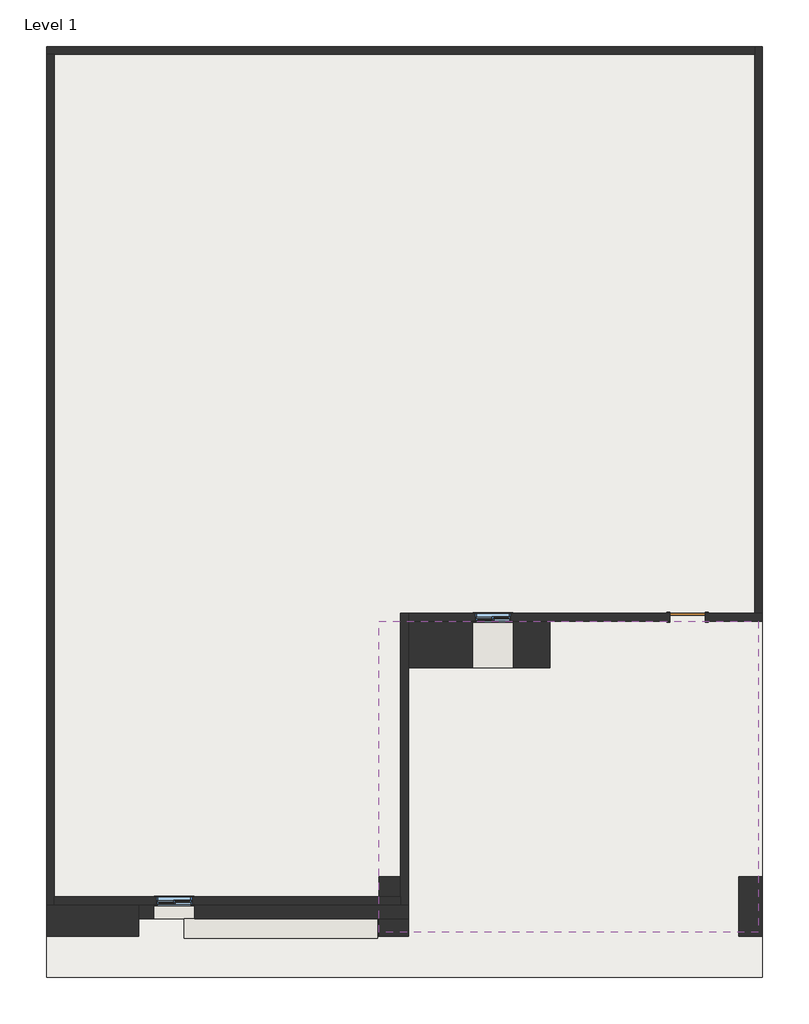
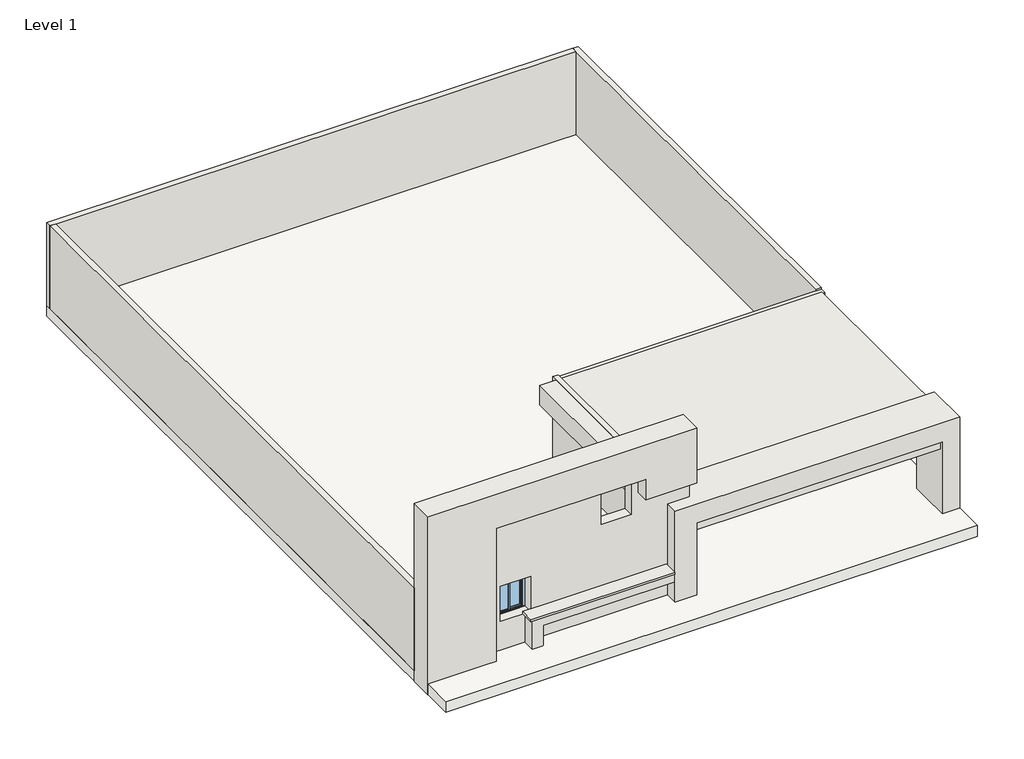
# One storey: 13 walls, 2 windows, 1 door, 1 slab.
"""IFC4 building model written with IfcOpenShell, lengths in millimetres."""

from ifc_helpers import new_model, si_unit, frame, origin, place, context, project, spatial, polyline, outline, extrude, faceted_brep, transform, mapped, element, save
from components import m_single_flush_0915_x_2134mm_6a9e8738, walls_1_walls_1_0e52aedd, walls_2_walls_2_fb44fb4a, walls_3_walls_3_d266139f, walls_4_walls_4_c70d8470, walls_5_walls_5_db9c16c0, walls_6_walls_6_9121aec3, walls_7_walls_7_ca1172f2, window_242facca

model = new_model("IFC4")

# Units and contexts
model_context = context("Model", 3, world=origin())
ifc_project = project(units=[si_unit("LENGTHUNIT", "METRE", prefix="MILLI")], contexts=[model_context])

# Site, building, storey
site = spatial("IfcSite", under=ifc_project)
building = spatial("IfcBuilding", under=site)
storey = spatial("IfcBuildingStorey", under=building, Name="Level 1", Elevation=0.0)

# Door
placement = place(None, origin())
m_single_flush_0915_x_2134mm_shape = m_single_flush_0915_x_2134mm_6a9e8738(model_context)
element("IfcDoor", 1, ObjectType="M_Single-Flush : 0915 x 2134mm", at=placement, inside=storey, context=model_context, shape_type="MappedRepresentation", body=[
    mapped(m_single_flush_0915_x_2134mm_shape, transform((-1283.2019361, 809.3437087, 0.0), x_axis=(1.0, 0.0, 0.0), y_axis=(0.0, 1.0, 0.0), z_axis=(0.0, 0.0, 1.0))),
])

# Slab
element("IfcSlab", 2, ObjectType="Generic Floor - 400mm", at=placement, inside=storey, context=model_context, shape_type="SweptSolid", body=[
    extrude(outline(polyline([(645.5980639, 15539.7437087), (645.5980639, -8487.0562913), (-17842.4019361, -8487.0562913), (-17842.4019361, 15539.7437087), (645.5980639, 15539.7437087)])), frame((0.0, 0.0, -400.0), z_axis=(0.0, 0.0, 1.0), x_axis=(1.0, 0.0, 0.0)), (0.0, 0.0, 1.0), 400.0),
])

# Walls
element("IfcWall", 3, ObjectType="Generic - 200mm", at=placement, inside=storey, context=model_context, shape_type="Brep", body=[
    faceted_brep([(-17842.4019361, 15339.7437087, 0.0), (-17642.4019361, 15339.7437087, 0.0), (445.5980639, 15339.7437087, 0.0), (445.5980639, 15339.7437087, 3048.0), (-17642.4019361, 15339.7437087, 3048.0), (-17842.4019361, 15339.7437087, 3048.0), (-17842.4019361, 15539.7437087, 0.0), (-17842.4019361, 15539.7437087, 3048.0), (445.5980639, 15539.7437087, 3048.0), (445.5980639, 15539.7437087, 0.0)], [[[0, 1, 2, 3, 4, 5]], [[6, 7, 8, 9]], [[2, 1, 0, 6, 9]], [[5, 4, 3, 8, 7]], [[0, 5, 7, 6]], [[3, 2, 9, 8]]]),
])
element("IfcWall", 4, ObjectType="Generic - 200mm", at=placement, inside=storey, context=model_context, shape_type="Brep", body=[
    faceted_brep([(-17642.4019361, -6605.8562913, 0.0), (-17642.4019361, -6405.8562913, 0.0), (-17642.4019361, 15339.7437087, 0.0), (-17642.4019361, 15339.7437087, 3048.0), (-17642.4019361, -6405.8562913, 3048.0), (-17642.4019361, -6605.8562913, 3048.0), (-17842.4019361, -6605.8562913, 0.0), (-17842.4019361, -6605.8562913, 3048.0), (-17842.4019361, 15339.7437087, 3048.0), (-17842.4019361, 15339.7437087, 0.0)], [[[0, 1, 2, 3, 4, 5]], [[6, 7, 8, 9]], [[2, 1, 0, 6, 9]], [[5, 4, 3, 8, 7]], [[0, 5, 7, 6]], [[3, 2, 9, 8]]]),
])
element("IfcWall", 5, ObjectType="Generic - 200mm", at=placement, inside=storey, context=model_context, shape_type="SweptSolid", body=[
    extrude(outline(polyline([(0.0, -8698.4019361), (3048.0, -8698.4019361), (3048.0, -17642.4019361), (0.0, -17642.4019361), (0.0, -8698.4019361)]), holes=[polyline([(2270.7381187, -14999.2019361), (2270.7381187, -14084.8019361), (1051.5381187, -14084.8019361), (1051.5381187, -14999.2019361), (2270.7381187, -14999.2019361)])]), frame((0.0, -6605.8562913, 0.0), z_axis=(0.0, 1.0, 0.0), x_axis=(0.0, 0.0, 1.0)), (0.0, 0.0, 1.0), 200.0),
])
element("IfcWall", 6, ObjectType="Generic - 200mm", at=placement, inside=storey, context=model_context, shape_type="Brep", body=[
    faceted_brep([(445.5980639, 15539.7437087, 0.0), (445.5980639, 15339.7437087, 0.0), (445.5980639, 909.3437087, 0.0), (445.5980639, 909.3437087, 3048.0), (445.5980639, 15339.7437087, 3048.0), (445.5980639, 15539.7437087, 3048.0), (645.5980639, 15539.7437087, 0.0), (645.5980639, 15539.7437087, 3048.0), (645.5980639, 909.3437087, 3048.0), (645.5980639, 909.3437087, 2994.8705823), (645.5980639, 909.3437087, 0.0)], [[[0, 1, 2, 3, 4, 5]], [[6, 7, 8, 9, 10]], [[2, 1, 0, 6, 10]], [[5, 4, 3, 8, 7]], [[0, 5, 7, 6]], [[3, 2, 10, 9, 8]]]),
])
element("IfcWall", 7, ObjectType="Generic - 200mm", at=placement, inside=storey, context=model_context, shape_type="Brep", body=[
    faceted_brep([(-8498.4019361, -6605.8562913, 0.0), (-8498.4019361, 709.3437087, 0.0), (-8498.4019361, 909.3437087, 0.0), (-8498.4019361, 909.3437087, 2994.8705823), (-8498.4019361, 909.3437087, 3048.0), (-8498.4019361, -6605.8562913, 3048.0), (-8698.4019361, -6605.8562913, 0.0), (-8698.4019361, -6605.8562913, 3048.0), (-8698.4019361, -6405.8562913, 3048.0), (-8698.4019361, 909.3437087, 3048.0), (-8698.4019361, 909.3437087, 0.0), (-8698.4019361, -6405.8562913, 0.0)], [[[0, 1, 2, 3, 4, 5]], [[6, 7, 8, 9, 10, 11]], [[2, 1, 0, 6, 11, 10]], [[5, 4, 9, 8, 7]], [[4, 3, 2, 10, 9]], [[0, 5, 7, 6]]]),
])
element("IfcWall", 8, ObjectType="Generic - 200mm", at=placement, inside=storey, context=model_context, shape_type="Brep", body=[
    faceted_brep([(-825.7019361, 709.3437087, 2134.0), (-825.7019361, 709.3437087, 0.0), (645.5980639, 709.3437087, 0.0), (645.5980639, 709.3437087, 2994.8705823), (-8498.4019361, 709.3437087, 2994.8705823), (-8498.4019361, 709.3437087, 0.0), (-1740.7019361, 709.3437087, 0.0), (-1740.7019361, 709.3437087, 2134.0), (-6769.6019361, 709.3437087, 1828.8), (-5855.2019361, 709.3437087, 1828.8), (-5855.2019361, 709.3437087, 609.6), (-6769.6019361, 709.3437087, 609.6), (645.5980639, 909.3437087, 0.0), (445.5980639, 909.3437087, 0.0), (-825.7019361, 909.3437087, 0.0), (-825.7019361, 909.3437087, 2134.0), (-1740.7019361, 909.3437087, 2134.0), (-1740.7019361, 909.3437087, 0.0), (-8498.4019361, 909.3437087, 0.0), (-8498.4019361, 909.3437087, 2994.8705823), (645.5980639, 909.3437087, 2994.8705823), (-6769.6019361, 909.3437087, 1828.8), (-6769.6019361, 909.3437087, 609.6), (-5855.2019361, 909.3437087, 609.6), (-5855.2019361, 909.3437087, 1828.8)], [[[0, 1, 2, 3, 4, 5, 6, 7], [8, 9, 10, 11]], [[12, 13, 14, 15, 16, 17, 18, 19, 20], [21, 22, 23, 24]], [[6, 5, 18, 17]], [[2, 1, 14, 13, 12]], [[4, 3, 20, 19]], [[5, 4, 19, 18]], [[3, 2, 12, 20]], [[15, 14, 1, 0]], [[16, 15, 0, 7]], [[17, 16, 7, 6]], [[22, 21, 8, 11]], [[23, 22, 11, 10]], [[24, 23, 10, 9]], [[21, 24, 9, 8]]]),
])
walls_1_walls_1_shape = walls_1_walls_1_0e52aedd(model_context)
element("IfcWall", 9, ObjectType="Walls 1 : Walls 1", at=placement, inside=storey, context=model_context, shape_type="MappedRepresentation", body=[
    mapped(walls_1_walls_1_shape, transform((0.0, 0.0, 0.0), x_axis=(1.0, 0.0, 0.0), y_axis=(0.0, 1.0, 0.0), z_axis=(0.0, 0.0, 1.0))),
])
walls_2_walls_2_shape = walls_2_walls_2_fb44fb4a(model_context)
element("IfcWall", 10, ObjectType="Walls 2 : Walls 2", at=placement, inside=storey, context=model_context, shape_type="MappedRepresentation", body=[
    mapped(walls_2_walls_2_shape, transform((0.0, 0.0, 0.0), x_axis=(1.0, 0.0, 0.0), y_axis=(0.0, 1.0, 0.0), z_axis=(0.0, 0.0, 1.0))),
])
walls_3_walls_3_shape = walls_3_walls_3_d266139f(model_context)
element("IfcWall", 11, ObjectType="Walls 3 : Walls 3", at=placement, inside=storey, context=model_context, shape_type="MappedRepresentation", body=[
    mapped(walls_3_walls_3_shape, transform((0.0, 0.0, 0.0), x_axis=(1.0, 0.0, 0.0), y_axis=(0.0, 1.0, 0.0), z_axis=(0.0, 0.0, 1.0))),
])
walls_4_walls_4_shape = walls_4_walls_4_c70d8470(model_context)
element("IfcWall", 12, ObjectType="Walls 4 : Walls 4", at=placement, inside=storey, context=model_context, shape_type="MappedRepresentation", body=[
    mapped(walls_4_walls_4_shape, transform((0.0, 0.0, 0.0), x_axis=(1.0, 0.0, 0.0), y_axis=(0.0, 1.0, 0.0), z_axis=(0.0, 0.0, 1.0))),
])
walls_5_walls_5_shape = walls_5_walls_5_db9c16c0(model_context)
element("IfcWall", 13, ObjectType="Walls 5 : Walls 5", at=placement, inside=storey, context=model_context, shape_type="MappedRepresentation", body=[
    mapped(walls_5_walls_5_shape, transform((0.0, 0.0, 0.0), x_axis=(1.0, 0.0, 0.0), y_axis=(0.0, 1.0, 0.0), z_axis=(0.0, 0.0, 1.0))),
])
walls_6_walls_6_shape = walls_6_walls_6_9121aec3(model_context)
element("IfcWall", 14, ObjectType="Walls 6 : Walls 6", at=placement, inside=storey, context=model_context, shape_type="MappedRepresentation", body=[
    mapped(walls_6_walls_6_shape, transform((0.0, 0.0, 0.0), x_axis=(1.0, 0.0, 0.0), y_axis=(0.0, 1.0, 0.0), z_axis=(0.0, 0.0, 1.0))),
])
walls_7_walls_7_shape = walls_7_walls_7_ca1172f2(model_context)
element("IfcWall", 15, ObjectType="Walls 7 : Walls 7", at=placement, inside=storey, context=model_context, shape_type="MappedRepresentation", body=[
    mapped(walls_7_walls_7_shape, transform((-29.7681082, 0.0, 0.0), x_axis=(1.0, 0.0, 0.0), y_axis=(0.0, 1.0, 0.0), z_axis=(0.0, 0.0, 1.0))),
])

# Windows
window_shape = window_242facca(model_context)
element("IfcWindow", 16, ObjectType="Slider with Trim : 36\" x 48\"", at=placement, inside=storey, context=model_context, shape_type="MappedRepresentation", body=[
    mapped(window_shape, transform((-14542.0019361, -6505.8562913, 137.1381187), x_axis=(-1.0, 0.0, 0.0), y_axis=(0.0, -1.0, 0.0), z_axis=(0.0, 0.0, 1.0))),
])
element("IfcWindow", 17, ObjectType="Slider with Trim : 36\" x 48\"", at=placement, inside=storey, context=model_context, shape_type="MappedRepresentation", body=[
    mapped(window_shape, transform((-6312.4019361, 809.3437087, -304.8), x_axis=(-1.0, 0.0, 0.0), y_axis=(0.0, -1.0, 0.0), z_axis=(0.0, 0.0, 1.0))),
])

save(model, "model.ifc")

# Revit data of these elements
# Type "M_Single-Flush : 0915 x 2134mm"
#   Type Mark = "15"
#   Thickness = 0' - 2.00787"
#   Height = 7' - 0.01575"
#   Trim Projection Ext = 0' - 0.98425"
#   Trim Projection Int = 0' - 0.98425"
#   Trim Width = 0' - 2.99213"
#   Width = 3' - 0.02362"
#   Door Material = Door - Panel
#   Frame Material = Door - Frame
#   Function = (empty or 0)
#   Wall Closure = (empty or 0)
# Type "Generic Floor - 400mm"
#   Function = 0
#   Layers, outside or top first: 1' - 3.74803" no material (function 1)
# Type "Generic - 200mm"
#   Layers, outside or top first: 0' - 7.87402" no material (function 1)
# Type "Slider with Trim : 36\" x 48\""
#   Type Mark = "19"
#   Construction Type Id = "GSP4R"
#   Assembly Code = "B2020100"
#   Analytic Construction = "1/8 in Pilkington single glazing"
#   Visual Light Transmittance = 0.9
#   Solar Heat Gain Coefficient = 0.78
#   Heat Transfer Coefficient (U) = 3.6886 W/(m²·K)
#   Height = 4' - 0"
#   Default Sill Height = 3' - 0"
#   Trim Projection - Ext. = 0' - 0 3/4"
#   Trim Projection - Int. = 0' - 0 3/4"
#   Trim Width - Exterior = 0' - 3 1/2"
#   Trim Width - Interior = 0' - 3 1/2"
#   Width = 3' - 0"
#   Window Inset = 0' - 0 3/4"
#   Define Thermal Properties by = 1
#   Glass Pane Material = Glass
#   Sash Material = Sash
#   Trim Exterior Material = Trim
#   Trim Interior Material = Trim
#   Wall Closure = (empty or 0)
# Element 1 (IfcDoor, "M_Single-Flush : 0915 x 2134mm")
#   Phase Created = New Construction
#   Materials on its faces: "Door - Frame", "Door - Panel"
# Element 2 (IfcSlab, "Generic Floor - 400mm")
#   Height Offset From Level = 0' - 0"
#   Phase Created = New Construction
#   Materials on its faces: "Default Roof"
# Elements 3, 4, 5, 6, 7 (IfcWall, "Generic - 200mm")
#   Top Offset = 0' - 0"
#   Base Offset = 0' - 0"
#   Unconnected Height = 10' - 0"
#   wall height = 10' - 0"
#   Phase Created = New Construction
#   Base Constraint = Level 1
#   Materials on its faces: "Default Wall"
# Element 8 (IfcWall, "Generic - 200mm")
#   Top Offset = 0' - 0"
#   Base Offset = 0' - 0"
#   Unconnected Height = 9' - 9.90829"
#   wall height = 9' - 9.90829"
#   Phase Created = New Construction
#   Base Constraint = Level 1
#   Materials on its faces: "Default Wall"
# Element 9 (IfcWall, "Walls 1 : Walls 1")
#   Phase Created = New Construction
#   Materials on its faces: "Default Wall"
# Element 10 (IfcWall, "Walls 2 : Walls 2")
#   Phase Created = New Construction
#   Materials on its faces: "Default Wall"
# Element 11 (IfcWall, "Walls 3 : Walls 3")
#   Phase Created = New Construction
#   Materials on its faces: "Default Wall"
# Element 12 (IfcWall, "Walls 4 : Walls 4")
#   Phase Created = New Construction
#   Materials on its faces: "Default Wall"
# Element 13 (IfcWall, "Walls 5 : Walls 5")
#   Phase Created = New Construction
#   Materials on its faces: "Default Wall"
# Element 14 (IfcWall, "Walls 6 : Walls 6")
#   Phase Created = New Construction
#   Materials on its faces: "Default Wall"
# Element 15 (IfcWall, "Walls 7 : Walls 7")
#   Phase Created = New Construction
#   Materials on its faces: "Default Wall"
# Element 16 (IfcWindow, "Slider with Trim : 36\" x 48\"")
#   Mark = "7"
#   Phase Created = New Construction
#   Materials on its faces: "Sash", "Trim", "Glass"
# Element 17 (IfcWindow, "Slider with Trim : 36\" x 48\"")
#   Mark = "8"
#   Phase Created = New Construction
#   Materials on its faces: "Sash", "Trim", "Glass"
# Materials
#   "Door - Panel": class "Wood", colour RGB 114 82 51, transparency 0
#   "Door - Frame": colour RGB 153 76 43, transparency 0
#   "Glass": class "Glass", colour RGB 218 227 224, transparency 0.85, Description = "Soda Lime Glass", Cost = 0
#   "Sash": class "Wood", colour RGB 136 99 55, transparency 0
#   "Trim": class "Wood", colour RGB 224 178 126, transparency 0
#   "Default Roof": colour RGB 80 80 80, transparency 0
#   "Default Wall": colour RGB 80 80 80, transparency 0
